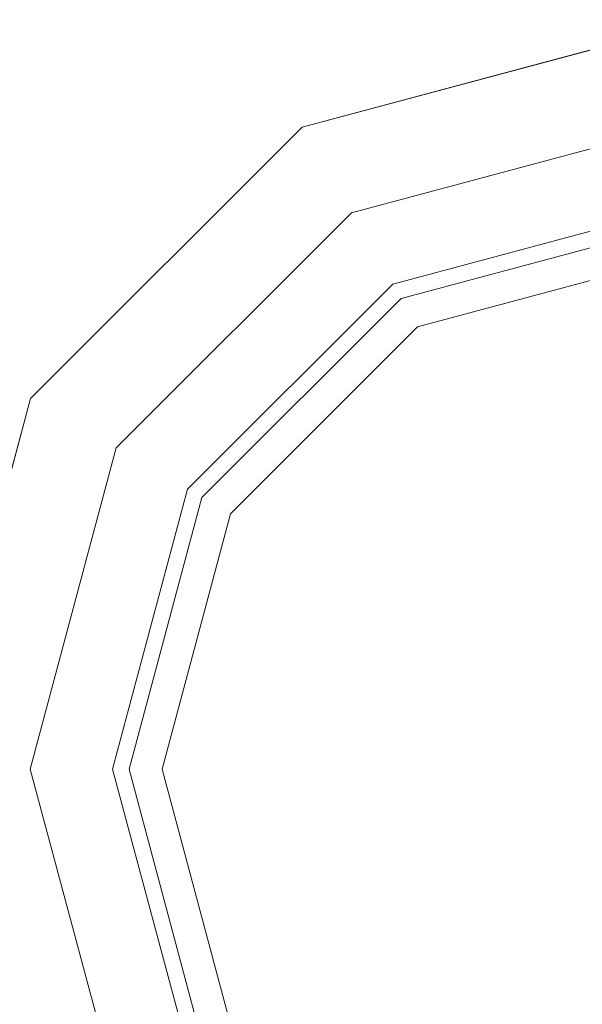
# Model space of a CAD drawing. Units: inches. Extents: x 375 to 1122, y 27 to 1069.
# Tile 112 of 155: x 734.892 to 739.094, y 867.512 to 874.871. Entities that reach past the tile are written whole.
import ezdxf

# ---------------------------------------------------------------- set-up
doc = ezdxf.new("R2010")
doc.units = ezdxf.units.IN
doc.layers.add('A-ANNO-DIMS', color=2, linetype='Continuous', lineweight=18)
doc.layers.add('Furniture', color=30, linetype='Continuous', lineweight=18)
doc.styles.get("Standard").update_dxf_attribs({"font": 'arial.ttf'})
doc.dimstyles.new('ISO-25', dxfattribs={"dimtxt": 12, "dimasz": 2.5, "dimexe": 1.5, "dimexo": 1.5, "dimtad": 1, "dimdec": 1, "dimlunit": 3, "dimtxsty": 'Standard', "dimblk": 'ARCHTICK', "dimcen": 2.5, "dimadec": 0, "dimazin": 0, "dimtfac": 1, "dimtdec": 1, "dimtmove": 0, "dimatfit": 3, "dimfxl": 1.5, "dimfxlon": 1, "dimarcsym": 0})

# ---------------------------------------------------------------- blocks, each defined once
blk = doc.blocks.new('A$C403C54AD')
at = {"linetype": 'ByBlock', "invisible_edges": 5}
for points in [[(1.58798, 1.37069, -0.02349), (1.60645, 1.37069, -0.02349), (1.62254, 1.31066, -0.02349), (1.60654, 1.30143, -0.02349)], [(1.62185, 1.37069, -0.03734), (1.58798, 1.37069, -0.02811), (1.60654, 1.30143, -0.02811), (1.63587, 1.31836, -0.03734)], [(1.60645, 1.37069, -0.02349), (1.62492, 1.37069, -0.02965), (1.63853, 1.3199, -0.02965), (1.62254, 1.31066, -0.02349)], [(1.63108, 1.37069, -0.04658), (1.62185, 1.37069, -0.03734), (1.63587, 1.31836, -0.03734), (1.64387, 1.32297, -0.04658)], [(1.62492, 1.37069, -0.02965), (1.72651, 1.37069, -0.02965), (1.72651, 1.37069, -0.02965), (1.63853, 1.3199, -0.02965)], [(1.63853, 1.3199, -0.02965), (1.72651, 1.37069, -0.02965), (1.72651, 1.37069, -0.02965), (1.67572, 1.28271, -0.02965)], [(1.67572, 1.28271, -0.02965), (1.72651, 1.37069, -0.02965), (1.72651, 1.37069, -0.02965), (1.72651, 1.2691, -0.02965)], [(1.72651, 1.2691, -0.02965), (1.72651, 1.37069, -0.02965), (1.72651, 1.37069, -0.02965), (1.7773, 1.28271, -0.02965)], [(1.81449, 1.3199, -0.02965), (1.72651, 1.37069, -0.02965), (1.72651, 1.37069, -0.02965), (1.8281, 1.37069, -0.02965)], [(1.7773, 1.28271, -0.02965), (1.72651, 1.37069, -0.02965), (1.72651, 1.37069, -0.02965), (1.81449, 1.3199, -0.02965)], [(1.64387, 1.32297, -0.04658), (1.63587, 1.31836, -0.03734), (1.67418, 1.28005, -0.03734), (1.6788, 1.28804, -0.04658)], [(1.62254, 1.31066, -0.02349), (1.63853, 1.3199, -0.02965), (1.67572, 1.28271, -0.02965), (1.66648, 1.26672, -0.02349)], [(1.63587, 1.31836, -0.03734), (1.60654, 1.30143, -0.02811), (1.65725, 1.25072, -0.02811), (1.67418, 1.28005, -0.03734)], [(1.60654, 1.30143, -0.02349), (1.62254, 1.31066, -0.02349), (1.66648, 1.26672, -0.02349), (1.65725, 1.25072, -0.02349)], [(1.6788, 1.28804, -0.04658), (1.67418, 1.28005, -0.03734), (1.72651, 1.26602, -0.03734), (1.72651, 1.27526, -0.04658)], [(1.72651, 1.27526, -0.04658), (1.72651, 1.26602, -0.03734), (1.77884, 1.28005, -0.03734), (1.77423, 1.28804, -0.04658)], [(1.66648, 1.26672, -0.02349), (1.67572, 1.28271, -0.02965), (1.72651, 1.2691, -0.02965), (1.72651, 1.25063, -0.02349)], [(1.72651, 1.25063, -0.02349), (1.72651, 1.2691, -0.02965), (1.7773, 1.28271, -0.02965), (1.78654, 1.26672, -0.02349)], [(1.67418, 1.28005, -0.03734), (1.65725, 1.25072, -0.02811), (1.72651, 1.23216, -0.02811), (1.72651, 1.26602, -0.03734)], [(1.72651, 1.26602, -0.03734), (1.72651, 1.23216, -0.02811), (1.79578, 1.25072, -0.02811), (1.77884, 1.28005, -0.03734)], [(1.65725, 1.25072, -0.02349), (1.66648, 1.26672, -0.02349), (1.72651, 1.25063, -0.02349), (1.72651, 1.23216, -0.02349)], [(1.72651, 1.23216, -0.02349), (1.72651, 1.25063, -0.02349), (1.78654, 1.26672, -0.02349), (1.79578, 1.25072, -0.02349)]]:
    blk.add_3dface(points, dxfattribs=at)
at = {"linetype": 'ByBlock'}
for points in [[(1.58798, 1.37069, -0.02811), (1.58798, 1.37069, -0.02349), (1.60654, 1.30143, -0.02349), (1.60654, 1.30143, -0.02811)], [(1.60654, 1.30143, -0.02811), (1.60654, 1.30143, -0.02349), (1.65725, 1.25072, -0.02349), (1.65725, 1.25072, -0.02811)], [(1.65725, 1.25072, -0.02811), (1.65725, 1.25072, -0.02349), (1.72651, 1.23216, -0.02349), (1.72651, 1.23216, -0.02811)], [(1.72651, 1.23216, -0.02811), (1.72651, 1.23216, -0.02349), (1.79578, 1.25072, -0.02349), (1.79578, 1.25072, -0.02811)]]:
    blk.add_3dface(points, dxfattribs=at)
blk = doc.blocks.new('_ArchTick')
at = {"color": 0, "linetype": 'ByBlock', "const_width": 0.15}
blk.add_lwpolyline([(-0.5, -0.5), (0.5, 0.5)], dxfattribs=at)
blk = doc.blocks.new('*D85')
at = {"layer": 'A-ANNO-DIMS', "color": 0, "lineweight": -2, "transparency": 16777216}
for p, q in [((401.5073, 868.5277), (398.5073, 868.5277)), ((400.0073, 814.5277), (400.0073, 868.5277)), ((401.5073, 814.5277), (398.5073, 814.5277))]:
    blk.add_line(p, q, dxfattribs=at)
at = {"layer": 'Defpoints', "color": 0, "transparency": 16777216}
for p in [(400.0073, 868.5277), (845.0073, 868.5277), (845.0073, 814.5277)]:
    blk.add_point(p, dxfattribs=at)
at = {"layer": 'A-ANNO-DIMS', "color": 0, "lineweight": -2, "transparency": 16777216, "xscale": 2.5, "yscale": 2.5, "zscale": 2.5}
for p, rotation in [((400.0073, 868.5277), 90), ((400.0073, 814.5277), 270)]:
    blk.add_blockref('_ArchTick', p, dxfattribs=dict(at, rotation=rotation))
at = {"layer": 'A-ANNO-DIMS', "color": 0, "transparency": 16777216, "insert": (393.2555, 841.5277), "char_height": 12, "attachment_point": 5, "rotation": 90}
blk.add_mtext('4\'-6"', dxfattribs=at)
blk = doc.blocks.new('*D88')
at = {"layer": 'A-ANNO-DIMS', "color": 0, "lineweight": -2, "transparency": 16777216}
for p, q in [((731.0073, 1052.5277), (731.0073, 1055.5277)), ((854.0073, 1052.5277), (854.0073, 1055.5277)), ((731.0073, 1054.0277), (854.0073, 1054.0277))]:
    blk.add_line(p, q, dxfattribs=at)
at = {"layer": 'Defpoints', "color": 0, "transparency": 16777216}
for p in [(854.0073, 1054.0277), (731.0073, 502.5277), (854.0073, 502.5277)]:
    blk.add_point(p, dxfattribs=at)
at = {"layer": 'A-ANNO-DIMS', "color": 0, "lineweight": -2, "transparency": 16777216, "xscale": 2.5, "yscale": 2.5, "zscale": 2.5, "rotation": 180}
blk.add_blockref('_ArchTick', (731.0073, 1054.0277), dxfattribs=at)
at = {"layer": 'A-ANNO-DIMS', "color": 0, "lineweight": -2, "transparency": 16777216, "xscale": 2.5, "yscale": 2.5, "zscale": 2.5}
blk.add_blockref('_ArchTick', (854.0073, 1054.0277), dxfattribs=at)
at = {"layer": 'A-ANNO-DIMS', "color": 0, "transparency": 16777216, "insert": (792.5073, 1060.7837), "char_height": 12, "attachment_point": 5}
blk.add_mtext('10\'-3"', dxfattribs=at)
blk = doc.blocks.new('*D91')
at = {"layer": 'A-ANNO-DIMS', "color": 0, "lineweight": -2, "transparency": 16777216}
for p, q in [((728.0073, 1052.5277), (728.0073, 1055.5277)), ((788.0073, 1052.5277), (788.0073, 1055.5277)), ((728.0073, 1054.0277), (788.0073, 1054.0277))]:
    blk.add_line(p, q, dxfattribs=at)
at = {"layer": 'Defpoints', "color": 0, "transparency": 16777216}
for p in [(788.0073, 1054.0277), (728.0073, 774.0277), (788.0073, 774.0277)]:
    blk.add_point(p, dxfattribs=at)
at = {"layer": 'A-ANNO-DIMS', "color": 0, "lineweight": -2, "transparency": 16777216, "xscale": 2.5, "yscale": 2.5, "zscale": 2.5, "rotation": 180}
blk.add_blockref('_ArchTick', (728.0073, 1054.0277), dxfattribs=at)
at = {"layer": 'A-ANNO-DIMS', "color": 0, "lineweight": -2, "transparency": 16777216, "xscale": 2.5, "yscale": 2.5, "zscale": 2.5}
blk.add_blockref('_ArchTick', (788.0073, 1054.0277), dxfattribs=at)
at = {"layer": 'A-ANNO-DIMS', "color": 0, "transparency": 16777216, "insert": (758.0073, 1060.7796), "char_height": 12, "attachment_point": 5}
blk.add_mtext('5\'-0"', dxfattribs=at)

msp = doc.modelspace()

# ---------------------------------------------------------------- block references
at = {"layer": 'Furniture', "xscale": 39.9918517141215, "yscale": 39.9918517141215, "zscale": 39.9918517141215, "rotation": 270}
msp.add_blockref('A$C403C54AD', (684.9549, 938.3156, 0.024), dxfattribs=at)

# ---------------------------------------------------------------- dimensions: what is measured, and where the dimension line sits
at = {"layer": 'A-ANNO-DIMS'}
for base, p1, p2, picture, middle in [((788.0073, 1054.0277), (728.0073, 774.0277), (788.0073, 774.0277), '*D91', (758.0073, 1060.7796)), ((854.0073, 1054.0277), (731.0073, 502.5277), (854.0073, 502.5277), '*D88', (792.5073, 1060.7837))]:
    dim = msp.add_linear_dim(base=base, p1=p1, p2=p2, dimstyle='ISO-25', override={"dimdec": 1, "dimlfac": 1, "dimrnd": 0, "dimzin": 1, "dimdsep": 46, "dimlunit": 4, "dimfrac": 2}, dxfattribs=at)
    dim.commit()
    dim.dimension.update_dxf_attribs({"geometry": picture, "text_midpoint": middle})
dim = msp.add_linear_dim(base=(400.0073, 868.5277), p1=(845.0073, 814.5277), p2=(845.0073, 868.5277), angle=90, dimstyle='ISO-25', override={"dimdec": 1, "dimlfac": 1, "dimrnd": 0, "dimzin": 1, "dimdsep": 46, "dimlunit": 4, "dimfrac": 2}, dxfattribs=at)
dim.commit()
dim.dimension.update_dxf_attribs({"geometry": '*D85', "text_midpoint": (393.2555, 841.5277)})

doc.saveas('drawing.dxf')
